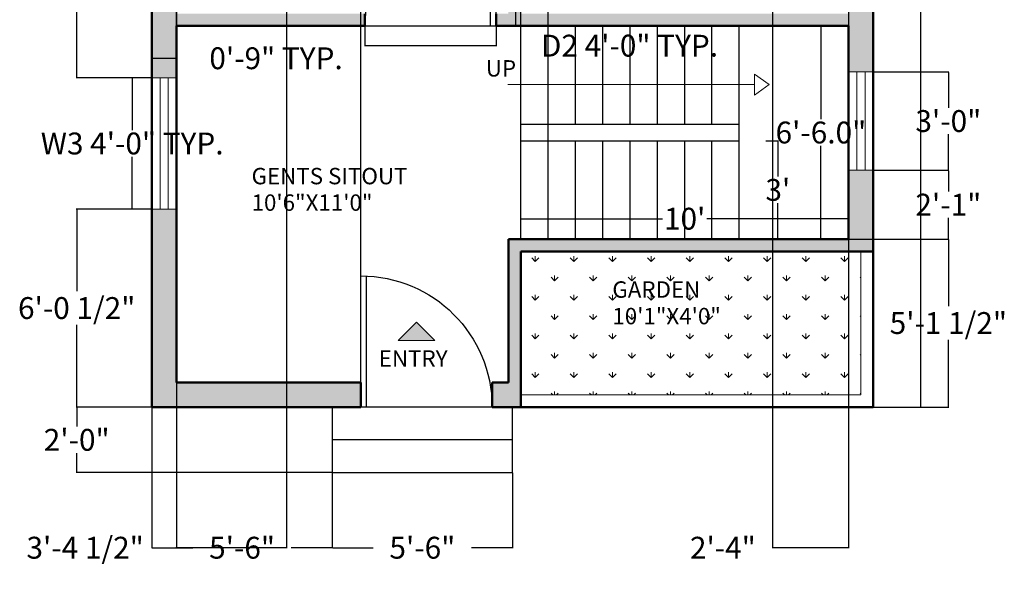
# Model space of a CAD drawing. Units: inches. Extents: x 23 to 387, y 67 to 650.
# Tile 1 of 3: x 23 to 384, y 67 to 272. Entities that reach past the tile are written whole.
import ezdxf

# ---------------------------------------------------------------- set-up
doc = ezdxf.new("R2010")
doc.units = ezdxf.units.IN
doc.header["$MEASUREMENT"] = 0
for name, color, linetype, lineweight in [('A-ANNO-DIMS', 4, 'Continuous', 18), ('A-ANNO-SYMB', 7, 'Continuous', 18), ('A-ANNO-TEXT', 4, 'Continuous', 18), ('A-AREA-IDEN', 4, 'Continuous', 25), ('A-DOOR', 41, 'Continuous', 25), ('A-FLOR-STRS', 215, 'Continuous', 25), ('A-GLAZ', 146, 'Continuous', 18), ('A-WALL', 240, 'Continuous', 50), ('A-WALL-PATT', 31, 'Continuous', 13), ('L-PLNT', 85, 'Continuous', 18), ('L-PLNT-PATT', 114, 'Continuous', 13)]:
    doc.layers.add(name, color=color, linetype=linetype, lineweight=lineweight)
doc.styles.get("Standard").update_dxf_attribs({"font": 'italic8.shx'})
doc.dimstyles.get("Standard").update_dxf_attribs({"dimtxt": 8, "dimasz": 0.18, "dimexe": 0.18, "dimexo": 0.0625, "dimgap": 0.09, "dimtad": 0, "dimtih": 1, "dimtoh": 1, "dimdec": 1, "dimzin": 0, "dimdsep": 46, "dimlunit": 3, "dimtxsty": 'Standard', "dimcen": 0.09, "dimadec": 0, "dimazin": 0, "dimtfac": 1, "dimtdec": 1, "dimtofl": 0, "dimtmove": 0, "dimatfit": 3, "dimfxl": 1, "dimtolj": 1, "dimtzin": 0, "dimarcsym": 0})

# ---------------------------------------------------------------- blocks, each defined once
blk = doc.blocks.new('*D1')
at = {"layer": 'A-ANNO-DIMS', "color": 0, "lineweight": -2, "transparency": 16777216}
for p, q in [((206.8, 199.3), (206.8, 199.68)), ((206.98, 199.5), (258.71, 199.5)), ((326.62, 199.5), (274.89, 199.5)), ((326.8, 199.3), (326.8, 199.68))]:
    blk.add_line(p, q, dxfattribs=at)
at = {"layer": 'A-ANNO-DIMS', "color": 0, "transparency": 16777216}
for points in [[(206.98, 199.53), (206.98, 199.47), (206.8, 199.5)], [(326.62, 199.53), (326.62, 199.47), (326.8, 199.5)]]:
    blk.add_solid(points, dxfattribs=at)
at = {"layer": 'Defpoints', "color": 0, "transparency": 16777216}
for p in [(206.8, 199.5), (206.8, 199.23), (326.8, 199.23)]:
    blk.add_point(p, dxfattribs=at)
at = {"layer": 'A-ANNO-DIMS', "color": 0, "transparency": 16777216, "insert": (266.8, 199.5), "char_height": 8, "attachment_point": 5}
blk.add_mtext("\\A1;10'", dxfattribs=at)
blk = doc.blocks.new('*D2')
at = {"layer": 'A-ANNO-DIMS', "color": 0, "lineweight": -2, "transparency": 16777216}
for p, q in [((316.66, 269.87), (316.66, 235.9)), ((316.72, 270.05), (316.84, 270.05)), ((316.66, 192.23), (316.66, 226.2)), ((316.72, 192.05), (316.84, 192.05))]:
    blk.add_line(p, q, dxfattribs=at)
at = {"layer": 'A-ANNO-DIMS', "color": 0, "transparency": 16777216}
for points in [[(316.63, 269.87), (316.69, 269.87), (316.66, 270.05)], [(316.63, 192.23), (316.69, 192.23), (316.66, 192.05)]]:
    blk.add_solid(points, dxfattribs=at)
at = {"layer": 'Defpoints', "color": 0, "transparency": 16777216}
for p in [(316.66, 270.05), (316.66, 270.05), (316.66, 192.05)]:
    blk.add_point(p, dxfattribs=at)
at = {"layer": 'A-ANNO-DIMS', "color": 0, "transparency": 16777216, "insert": (316.66, 231.05), "char_height": 8, "attachment_point": 5}
blk.add_mtext('\\A1;6\'-6.0"', dxfattribs=at)
blk = doc.blocks.new('*D3')
at = {"layer": 'A-ANNO-DIMS', "color": 0, "lineweight": -2, "transparency": 16777216}
for p, q in [((296.5, 228.05), (301.08, 228.05)), ((300.9, 227.87), (300.9, 214.9)), ((300.9, 192.23), (300.9, 205.2)), ((296.5, 192.05), (301.08, 192.05))]:
    blk.add_line(p, q, dxfattribs=at)
at = {"layer": 'A-ANNO-DIMS', "color": 0, "transparency": 16777216}
for points in [[(300.87, 227.87), (300.93, 227.87), (300.9, 228.05)], [(300.87, 192.23), (300.93, 192.23), (300.9, 192.05)]]:
    blk.add_solid(points, dxfattribs=at)
at = {"layer": 'Defpoints', "color": 0, "transparency": 16777216}
for p in [(296.44, 228.05), (300.9, 228.05), (296.44, 192.05)]:
    blk.add_point(p, dxfattribs=at)
at = {"layer": 'A-ANNO-DIMS', "color": 0, "transparency": 16777216, "insert": (300.9, 210.05), "char_height": 8, "attachment_point": 5}
blk.add_mtext("\\A1;3'", dxfattribs=at)
blk = doc.blocks.new('*D5')
at = {"layer": 'A-ANNO-DIMS', "color": 0, "lineweight": -2, "transparency": 16777216}
for p, q in [((335.86, 610.55), (353.42, 610.55)), ((353.24, 610.37), (353.24, 375.4)), ((353.24, 130.73), (353.24, 365.7)), ((335.86, 130.55), (353.42, 130.55))]:
    blk.add_line(p, q, dxfattribs=at)
at = {"layer": 'A-ANNO-DIMS', "color": 0, "transparency": 16777216}
for points in [[(353.21, 610.37), (353.27, 610.37), (353.24, 610.55)], [(353.21, 130.73), (353.27, 130.73), (353.24, 130.55)]]:
    blk.add_solid(points, dxfattribs=at)
at = {"layer": 'Defpoints', "color": 0, "transparency": 16777216}
for p in [(335.8, 610.55), (335.8, 130.55), (353.24, 130.55)]:
    blk.add_point(p, dxfattribs=at)
at = {"layer": 'A-ANNO-DIMS', "color": 0, "transparency": 16777216, "insert": (353.24, 370.55), "char_height": 8, "attachment_point": 5}
blk.add_mtext("\\A1;40'", dxfattribs=at)
blk = doc.blocks.new('DOOR-SWING-48IN')
for p, q in [((46, 0), (46, 47.96)), ((48, 0), (48, 48)), ((0, 0), (48, 0))]:
    blk.add_line(p, q)
blk.add_arc((48, 0), 48, 90, 180)
blk = doc.blocks.new('WIN-48IN')
for p, q in [((0, 0), (0, 48)), ((0, 48), (9, 48)), ((3, 0), (3, 48)), ((6, 0), (6, 48)), ((9, 48), (9, 0)), ((9, 0), (0, 0)), ((0, 0), (4.5, 0))]:
    blk.add_line(p, q)
blk = doc.blocks.new('*D16')
at = {"layer": 'A-ANNO-DIMS', "color": 0, "lineweight": -2, "transparency": 16777216}
for p, q in [((71.74, 251.04), (64.42, 251.04)), ((64.6, 250.86), (64.6, 231.89)), ((64.6, 203.22), (64.6, 222.19)), ((71.74, 203.04), (64.42, 203.04))]:
    blk.add_line(p, q, dxfattribs=at)
at = {"layer": 'A-ANNO-DIMS', "color": 0, "transparency": 16777216}
for points in [[(64.57, 250.86), (64.63, 250.86), (64.6, 251.04)], [(64.57, 203.22), (64.63, 203.22), (64.6, 203.04)]]:
    blk.add_solid(points, dxfattribs=at)
at = {"layer": 'Defpoints', "color": 0, "transparency": 16777216}
for p in [(64.6, 251.04), (71.8, 251.04), (71.8, 203.04)]:
    blk.add_point(p, dxfattribs=at)
at = {"layer": 'A-ANNO-DIMS', "color": 0, "transparency": 16777216, "insert": (64.6, 227.04), "char_height": 8, "attachment_point": 5}
blk.add_mtext('\\A1;W3 4\'-0" TYP.', dxfattribs=at)
blk = doc.blocks.new('*D17')
at = {"layer": 'A-ANNO-DIMS', "color": 0, "lineweight": -2, "transparency": 16777216}
for p, q in [((71.8, 251.1), (71.8, 258.42)), ((71.98, 258.24), (80.62, 258.24)), ((80.8, 251.1), (80.8, 258.42)), ((80.8, 258.24), (80.98, 258.24))]:
    blk.add_line(p, q, dxfattribs=at)
at = {"layer": 'A-ANNO-DIMS', "color": 0, "transparency": 16777216}
for points in [[(71.98, 258.27), (71.98, 258.21), (71.8, 258.24)], [(80.62, 258.27), (80.62, 258.21), (80.8, 258.24)]]:
    blk.add_solid(points, dxfattribs=at)
at = {"layer": 'Defpoints', "color": 0, "transparency": 16777216}
for p in [(80.8, 258.24), (71.8, 251.04), (80.8, 251.04)]:
    blk.add_point(p, dxfattribs=at)
at = {"layer": 'A-ANNO-DIMS', "color": 0, "transparency": 16777216, "insert": (117.26, 258.24), "char_height": 8, "attachment_point": 5}
blk.add_mtext('\\A1;0\'-9" TYP.', dxfattribs=at)
blk = doc.blocks.new('*D22')
at = {"layer": 'A-ANNO-DIMS', "color": 0, "lineweight": -2, "transparency": 16777216}
for p, q in [((149.76, 269.99), (149.76, 262.67)), ((197.76, 269.99), (197.76, 262.67)), ((149.94, 262.85), (197.58, 262.85)), ((197.76, 262.85), (197.94, 262.85))]:
    blk.add_line(p, q, dxfattribs=at)
at = {"layer": 'A-ANNO-DIMS', "color": 0, "transparency": 16777216}
for points in [[(149.94, 262.88), (149.94, 262.82), (149.76, 262.85)], [(197.58, 262.88), (197.58, 262.82), (197.76, 262.85)]]:
    blk.add_solid(points, dxfattribs=at)
at = {"layer": 'Defpoints', "color": 0, "transparency": 16777216}
for p in [(149.76, 270.05), (197.76, 270.05), (197.76, 262.85)]:
    blk.add_point(p, dxfattribs=at)
at = {"layer": 'A-ANNO-DIMS', "color": 0, "transparency": 16777216, "insert": (246.6, 262.85), "char_height": 8, "attachment_point": 5}
blk.add_mtext('\\A1;D2 4\'-0" TYP.', dxfattribs=at)
blk = doc.blocks.new('*D23')
at = {"layer": 'A-ANNO-DIMS', "color": 0, "lineweight": -2, "transparency": 16777216}
for p, q in [((197.82, 318.05), (205.14, 318.05)), ((204.96, 317.87), (204.96, 298.9)), ((204.96, 270.23), (204.96, 289.2)), ((197.82, 270.05), (205.14, 270.05))]:
    blk.add_line(p, q, dxfattribs=at)
at = {"layer": 'A-ANNO-DIMS', "color": 0, "transparency": 16777216}
for points in [[(204.93, 317.87), (204.99, 317.87), (204.96, 318.05)], [(204.93, 270.23), (204.99, 270.23), (204.96, 270.05)]]:
    blk.add_solid(points, dxfattribs=at)
at = {"layer": 'Defpoints', "color": 0, "transparency": 16777216}
for p in [(197.76, 318.05), (204.96, 318.05), (197.76, 270.05)]:
    blk.add_point(p, dxfattribs=at)
at = {"layer": 'A-ANNO-DIMS', "color": 0, "transparency": 16777216, "insert": (204.96, 294.05), "char_height": 8, "attachment_point": 5}
blk.add_mtext('\\A1;4\'-0" TYP.', dxfattribs=at)
blk = doc.blocks.new('*D24')
at = {"layer": 'A-ANNO-DIMS', "color": 0, "lineweight": -2, "transparency": 16777216}
for p, q in [((71.74, 130.55), (44.12, 130.55)), ((44.3, 130.37), (44.3, 123.4)), ((44.3, 106.73), (44.3, 113.7)), ((137.77, 106.55), (44.12, 106.55))]:
    blk.add_line(p, q, dxfattribs=at)
at = {"layer": 'A-ANNO-DIMS', "color": 0, "transparency": 16777216}
for points in [[(44.27, 130.37), (44.33, 130.37), (44.3, 130.55)], [(44.27, 106.73), (44.33, 106.73), (44.3, 106.55)]]:
    blk.add_solid(points, dxfattribs=at)
at = {"layer": 'Defpoints', "color": 0, "transparency": 16777216}
for p in [(44.3, 130.55), (71.8, 130.55), (137.83, 106.55)]:
    blk.add_point(p, dxfattribs=at)
at = {"layer": 'A-ANNO-DIMS', "color": 0, "transparency": 16777216, "insert": (44.3, 118.55), "char_height": 8, "attachment_point": 5}
blk.add_mtext('\\A1;2\'-0"', dxfattribs=at)
blk = doc.blocks.new('*D25')
at = {"layer": 'A-ANNO-DIMS', "color": 0, "lineweight": -2, "transparency": 16777216}
for p, q in [((137.83, 106.49), (137.83, 78.87)), ((203.79, 106.49), (203.79, 78.87)), ((138.01, 79.05), (152.81, 79.05)), ((203.61, 79.05), (188.8, 79.05))]:
    blk.add_line(p, q, dxfattribs=at)
at = {"layer": 'A-ANNO-DIMS', "color": 0, "transparency": 16777216}
for points in [[(138.01, 79.08), (138.01, 79.02), (137.83, 79.05)], [(203.61, 79.08), (203.61, 79.02), (203.79, 79.05)]]:
    blk.add_solid(points, dxfattribs=at)
at = {"layer": 'Defpoints', "color": 0, "transparency": 16777216}
for p in [(137.83, 106.55), (203.79, 106.55), (203.79, 79.05)]:
    blk.add_point(p, dxfattribs=at)
at = {"layer": 'A-ANNO-DIMS', "color": 0, "transparency": 16777216, "insert": (170.81, 79.05), "char_height": 8, "attachment_point": 5}
blk.add_mtext('\\A1;5\'-6"', dxfattribs=at)
blk = doc.blocks.new('*D26')
at = {"layer": 'A-ANNO-DIMS', "color": 0, "lineweight": -2, "transparency": 16777216}
for p, q in [((71.8, 130.49), (71.8, 78.87)), ((137.83, 106.49), (137.83, 78.87)), ((71.98, 79.05), (86.82, 79.05)), ((137.65, 79.05), (122.81, 79.05))]:
    blk.add_line(p, q, dxfattribs=at)
at = {"layer": 'A-ANNO-DIMS', "color": 0, "transparency": 16777216}
for points in [[(71.98, 79.08), (71.98, 79.02), (71.8, 79.05)], [(137.65, 79.08), (137.65, 79.02), (137.83, 79.05)]]:
    blk.add_solid(points, dxfattribs=at)
at = {"layer": 'Defpoints', "color": 0, "transparency": 16777216}
for p in [(71.8, 130.55), (137.83, 106.55), (137.83, 79.05)]:
    blk.add_point(p, dxfattribs=at)
at = {"layer": 'A-ANNO-DIMS', "color": 0, "transparency": 16777216, "insert": (104.82, 79.05), "char_height": 8, "attachment_point": 5}
blk.add_mtext('\\A1;5\'-6"', dxfattribs=at)
blk = doc.blocks.new('*D28')
at = {"layer": 'A-ANNO-DIMS', "color": 0, "lineweight": -2, "transparency": 16777216}
for p, q in [((71.74, 203.04), (44.12, 203.04)), ((44.3, 202.86), (44.3, 172.98)), ((44.3, 130.73), (44.3, 160.61)), ((71.74, 130.55), (44.12, 130.55))]:
    blk.add_line(p, q, dxfattribs=at)
at = {"layer": 'A-ANNO-DIMS', "color": 0, "transparency": 16777216}
for points in [[(44.27, 202.86), (44.33, 202.86), (44.3, 203.04)], [(44.27, 130.73), (44.33, 130.73), (44.3, 130.55)]]:
    blk.add_solid(points, dxfattribs=at)
at = {"layer": 'Defpoints', "color": 0, "transparency": 16777216}
for p in [(44.3, 203.04), (71.8, 203.04), (71.8, 130.55)]:
    blk.add_point(p, dxfattribs=at)
at = {"layer": 'A-ANNO-DIMS', "color": 0, "transparency": 16777216, "insert": (44.3, 166.79), "char_height": 8, "attachment_point": 5}
blk.add_mtext('\\A1;6\'-0 1/2"', dxfattribs=at)
blk = doc.blocks.new('*D31')
at = {"layer": 'A-ANNO-DIMS', "color": 0, "lineweight": -2, "transparency": 16777216}
for p, q in [((71.74, 322.2), (44.12, 322.2)), ((44.3, 322.02), (44.3, 291.47)), ((44.3, 251.22), (44.3, 281.76)), ((71.74, 251.04), (44.12, 251.04))]:
    blk.add_line(p, q, dxfattribs=at)
at = {"layer": 'A-ANNO-DIMS', "color": 0, "transparency": 16777216}
for points in [[(44.27, 322.02), (44.33, 322.02), (44.3, 322.2)], [(44.27, 251.22), (44.33, 251.22), (44.3, 251.04)]]:
    blk.add_solid(points, dxfattribs=at)
at = {"layer": 'Defpoints', "color": 0, "transparency": 16777216}
for p in [(71.8, 322.2), (44.3, 251.04), (71.8, 251.04)]:
    blk.add_point(p, dxfattribs=at)
at = {"layer": 'A-ANNO-DIMS', "color": 0, "transparency": 16777216, "insert": (44.3, 286.62), "char_height": 8, "attachment_point": 5}
blk.add_mtext('\\A1;5\'-11"', dxfattribs=at)
blk = doc.blocks.new('*D32')
at = {"layer": 'A-ANNO-DIMS', "color": 0, "lineweight": -2, "transparency": 16777216}
for p, q in [((335.86, 217.25), (363.48, 217.25)), ((363.3, 217.07), (363.3, 209.5)), ((363.3, 192.23), (363.3, 199.8)), ((326.86, 192.05), (363.48, 192.05))]:
    blk.add_line(p, q, dxfattribs=at)
at = {"layer": 'A-ANNO-DIMS', "color": 0, "transparency": 16777216}
for points in [[(363.27, 217.07), (363.33, 217.07), (363.3, 217.25)], [(363.27, 192.23), (363.33, 192.23), (363.3, 192.05)]]:
    blk.add_solid(points, dxfattribs=at)
at = {"layer": 'Defpoints', "color": 0, "transparency": 16777216}
for p in [(335.8, 217.25), (363.3, 217.25), (326.8, 192.05)]:
    blk.add_point(p, dxfattribs=at)
at = {"layer": 'A-ANNO-DIMS', "color": 0, "transparency": 16777216, "insert": (363.3, 204.65), "char_height": 8, "attachment_point": 5}
blk.add_mtext('\\A1;2\'-1"', dxfattribs=at)
blk = doc.blocks.new('*D36')
at = {"layer": 'A-ANNO-DIMS', "color": 0, "lineweight": -2, "transparency": 16777216}
for p, q in [((335.86, 253.25), (363.48, 253.25)), ((363.3, 253.07), (363.3, 240.11)), ((363.3, 217.43), (363.3, 230.4)), ((335.86, 217.25), (363.48, 217.25))]:
    blk.add_line(p, q, dxfattribs=at)
at = {"layer": 'A-ANNO-DIMS', "color": 0, "transparency": 16777216}
for points in [[(363.27, 253.07), (363.33, 253.07), (363.3, 253.25)], [(363.27, 217.43), (363.33, 217.43), (363.3, 217.25)]]:
    blk.add_solid(points, dxfattribs=at)
at = {"layer": 'Defpoints', "color": 0, "transparency": 16777216}
for p in [(335.8, 253.25), (335.8, 217.25), (363.3, 217.25)]:
    blk.add_point(p, dxfattribs=at)
at = {"layer": 'A-ANNO-DIMS', "color": 0, "transparency": 16777216, "insert": (363.3, 235.25), "char_height": 8, "attachment_point": 5}
blk.add_mtext('\\A1;3\'-0"', dxfattribs=at)
blk = doc.blocks.new('*D37')
at = {"layer": 'A-ANNO-DIMS', "color": 0, "lineweight": -2, "transparency": 16777216}
for p, q in [((80.8, 139.61), (80.8, 638.23)), ((80.98, 638.05), (81.51, 638.05)), ((148.12, 638.05), (147.59, 638.05)), ((148.3, 139.61), (148.3, 638.23))]:
    blk.add_line(p, q, dxfattribs=at)
at = {"layer": 'A-ANNO-DIMS', "color": 0, "transparency": 16777216}
for points in [[(80.98, 638.08), (80.98, 638.02), (80.8, 638.05)], [(148.12, 638.08), (148.12, 638.02), (148.3, 638.05)]]:
    blk.add_solid(points, dxfattribs=at)
at = {"layer": 'Defpoints', "color": 0, "transparency": 16777216}
for p in [(148.3, 638.05), (80.8, 139.55), (148.3, 139.55)]:
    blk.add_point(p, dxfattribs=at)
at = {"layer": 'A-ANNO-DIMS', "color": 0, "transparency": 16777216, "insert": (114.55, 638.05), "char_height": 8, "attachment_point": 5}
blk.add_mtext('\\A1;5\'-7 1/2"', dxfattribs=at)
blk = doc.blocks.new('*D39')
at = {"layer": 'A-ANNO-DIMS', "color": 0, "lineweight": -2, "transparency": 16777216}
for p, q in [((206.8, 192.11), (206.8, 638.23)), ((206.98, 638.05), (216.62, 638.05)), ((216.8, 192.11), (216.8, 638.23)), ((216.8, 638.05), (216.98, 638.05))]:
    blk.add_line(p, q, dxfattribs=at)
at = {"layer": 'A-ANNO-DIMS', "color": 0, "transparency": 16777216}
for points in [[(206.98, 638.08), (206.98, 638.02), (206.8, 638.05)], [(216.62, 638.08), (216.62, 638.02), (216.8, 638.05)]]:
    blk.add_solid(points, dxfattribs=at)
at = {"layer": 'Defpoints', "color": 0, "transparency": 16777216}
for p in [(216.8, 638.05), (206.8, 192.05), (216.8, 192.05)]:
    blk.add_point(p, dxfattribs=at)
at = {"layer": 'A-ANNO-DIMS', "color": 0, "transparency": 16777216, "insert": (237.64, 638.05), "char_height": 8, "attachment_point": 5}
blk.add_mtext('\\A1;0\'-10"', dxfattribs=at)
blk = doc.blocks.new('*D40')
at = {"layer": 'A-ANNO-DIMS', "color": 0, "lineweight": -2, "transparency": 16777216}
for p, q in [((80.8, 601.49), (80.8, 78.87)), ((121.14, 558.4), (121.14, 78.87)), ((80.8, 79.05), (80.62, 79.05)), ((120.96, 79.05), (80.98, 79.05))]:
    blk.add_line(p, q, dxfattribs=at)
at = {"layer": 'A-ANNO-DIMS', "color": 0, "transparency": 16777216}
for points in [[(80.98, 79.08), (80.98, 79.02), (80.8, 79.05)], [(120.96, 79.08), (120.96, 79.02), (121.14, 79.05)]]:
    blk.add_solid(points, dxfattribs=at)
at = {"layer": 'Defpoints', "color": 0, "transparency": 16777216}
for p in [(80.8, 601.55), (121.14, 558.46), (80.8, 79.05)]:
    blk.add_point(p, dxfattribs=at)
at = {"layer": 'A-ANNO-DIMS', "color": 0, "transparency": 16777216, "insert": (47.39, 79.05), "char_height": 8, "attachment_point": 5}
blk.add_mtext('\\A1;3\'-4 1/2"', dxfattribs=at)
blk = doc.blocks.new('*D43')
at = {"layer": 'A-ANNO-DIMS', "color": 0, "lineweight": -2, "transparency": 16777216}
for p, q in [((326.8, 601.49), (326.8, 78.87)), ((298.95, 586.36), (298.95, 78.87)), ((298.95, 79.05), (298.77, 79.05)), ((326.62, 79.05), (299.13, 79.05))]:
    blk.add_line(p, q, dxfattribs=at)
at = {"layer": 'A-ANNO-DIMS', "color": 0, "transparency": 16777216}
for points in [[(299.13, 79.08), (299.13, 79.02), (298.95, 79.05)], [(326.62, 79.08), (326.62, 79.02), (326.8, 79.05)]]:
    blk.add_solid(points, dxfattribs=at)
at = {"layer": 'Defpoints', "color": 0, "transparency": 16777216}
for p in [(326.8, 601.55), (298.95, 586.43), (298.95, 79.05)]:
    blk.add_point(p, dxfattribs=at)
at = {"layer": 'A-ANNO-DIMS', "color": 0, "transparency": 16777216, "insert": (280.78, 79.05), "char_height": 8, "attachment_point": 5}
blk.add_mtext('\\A1;2\'-4"', dxfattribs=at)
blk = doc.blocks.new('*D47')
at = {"layer": 'A-ANNO-DIMS', "color": 0, "lineweight": -2, "transparency": 16777216}
for p, q in [((326.86, 192.05), (363.48, 192.05)), ((363.3, 191.87), (363.3, 167.48)), ((363.3, 130.73), (363.3, 155.11)), ((335.86, 130.55), (363.48, 130.55))]:
    blk.add_line(p, q, dxfattribs=at)
at = {"layer": 'A-ANNO-DIMS', "color": 0, "transparency": 16777216}
for points in [[(363.27, 191.87), (363.33, 191.87), (363.3, 192.05)], [(363.27, 130.73), (363.33, 130.73), (363.3, 130.55)]]:
    blk.add_solid(points, dxfattribs=at)
at = {"layer": 'Defpoints', "color": 0, "transparency": 16777216}
for p in [(326.8, 192.05), (363.3, 192.05), (335.8, 130.55)]:
    blk.add_point(p, dxfattribs=at)
at = {"layer": 'A-ANNO-DIMS', "color": 0, "transparency": 16777216, "insert": (363.3, 161.3), "char_height": 8, "attachment_point": 5}
blk.add_mtext('\\A1;5\'-1 1/2"', dxfattribs=at)

msp = doc.modelspace()

# ---------------------------------------------------------------- hatches: boundary and pattern name
at = {"layer": 'A-ANNO-SYMB'}
h = msp.add_hatch(color=256, dxfattribs=at)
h.dxf.hatch_style = 1
h.paths.add_polyline_path([(168.68, 161.67), (161.99, 154.96), (168.68, 154.96), (175.36, 154.96)])
at = {"layer": 'A-WALL-PATT'}
h = msp.add_hatch(color=256, dxfattribs=at)
h.dxf.hatch_style = 1
h.paths.add_polyline_path([(80.8, 601.55), (168.85, 601.55), (168.85, 610.55), (71.8, 610.55), (71.8, 559.71), (80.8, 559.71)])
h.paths.add_polyline_path([(335.8, 610.55), (198.85, 610.55), (198.85, 601.55), (202.3, 601.55), (202.3, 481.55), (202.3, 465.05), (207.59, 465.05), (207.59, 469.55), (206.8, 469.55), (206.8, 601.55), (326.8, 601.55), (326.8, 570), (331.3, 570), (335.8, 570)])
h.paths.add_polyline_path([(335.8, 510), (326.8, 510), (326.8, 469.55), (249.59, 469.55), (249.59, 465.05), (250.3, 465.05), (250.3, 461.06), (254.8, 461.06), (254.8, 465.05), (326.8, 465.05), (326.8, 455.49), (335.8, 455.49)])
h.paths.add_polyline_path([(335.8, 425.49), (326.8, 425.49), (326.8, 414.55), (254.8, 414.55), (254.8, 431.06), (250.3, 431.06), (250.3, 414.55), (249.82, 414.55), (249.82, 410.05), (326.8, 410.05), (326.8, 362.57), (335.8, 362.57)])
h.paths.add_polyline_path([(335.8, 302.57), (326.8, 302.57), (326.8, 274.55), (206.8, 274.55), (206.8, 410.05), (207.82, 410.05), (207.82, 414.55), (202.3, 414.55), (202.3, 274.55), (197.76, 274.55), (197.76, 270.05), (326.8, 270.05), (326.8, 253.25), (335.8, 253.25)])
h.paths.add_polyline_path([(335.8, 217.25), (326.8, 217.25), (326.8, 192.05), (202.3, 192.05), (202.3, 139.55), (196.3, 139.55), (196.3, 130.55), (206.8, 130.55), (206.8, 187.55), (335.8, 187.55)])
h.paths.add_polyline_path([(80.8, 203.04), (71.8, 203.04), (71.8, 130.55), (148.3, 130.55), (148.3, 139.55), (80.8, 139.55)])
h.paths.add_polyline_path([(80.8, 322.2), (71.8, 322.2), (71.8, 251.04), (80.8, 251.04), (80.8, 270.05), (149.76, 270.05), (149.76, 274.55), (80.8, 274.55)])
h.paths.add_polyline_path([(80.8, 410.05), (133.3, 410.05), (133.3, 433.95), (128.8, 433.95), (128.8, 414.55), (80.8, 414.55), (80.8, 426.74), (71.8, 426.74), (71.8, 382.2), (80.8, 382.2)])
h.paths.add_polyline_path([(133.3, 479.05), (80.8, 479.05), (80.8, 511.71), (71.8, 511.71), (71.8, 456.74), (80.8, 456.74), (80.8, 474.55), (128.8, 474.55), (128.8, 469.95), (133.3, 469.95)])
h.paths.add_polyline_path([(82.53, 419.2), (134.1, 419.2), (134.1, 429.92), (82.53, 429.92)], flags=9)
at = {"layer": 'L-PLNT-PATT'}
h = msp.add_hatch(dxfattribs=at)
h.set_pattern_fill('GRASS', color=256, scale=10)
h.paths.add_polyline_path([(331.3, 187.55), (206.8, 187.55), (206.8, 135.05), (331.3, 135.05)])
h.paths.add_polyline_path([(238.84, 159.07), (292.13, 159.07), (292.13, 169.78), (238.84, 169.78)], flags=24)
h.paths.add_polyline_path([(238.84, 169.07), (281.55, 169.07), (281.55, 178.07), (238.84, 178.07)], flags=24)

# ---------------------------------------------------------------- linework, layer by layer
at = {"layer": 'A-ANNO-SYMB'}
for p, q in [((292.34, 248.57), (292.34, 252.44)), ((292.34, 252.44), (297.7, 248.57)), ((202.08, 248.57), (292.34, 248.57)), ((292.34, 248.57), (292.34, 244.7)), ((292.34, 244.7), (297.7, 248.57)), ((161.99, 154.96), (168.68, 161.67)), ((175.36, 154.96), (168.68, 161.67)), ((168.68, 154.96), (161.99, 154.96)), ((168.68, 154.96), (175.36, 154.96))]:
    msp.add_line(p, q, dxfattribs=at)
at = {"layer": 'A-FLOR-STRS'}
for p, q in [((206.8, 192.05), (206.8, 270.05)), ((216.8, 234.05), (216.8, 270.05)), ((226.8, 234.05), (226.8, 270.05)), ((236.8, 234.05), (236.8, 270.05)), ((246.8, 234.05), (246.8, 270.05)), ((256.8, 234.05), (256.8, 270.05)), ((266.8, 234.05), (266.8, 270.05)), ((276.8, 234.05), (276.8, 270.05)), ((286.8, 192.05), (286.8, 270.05)), ((206.8, 234.05), (286.8, 234.05)), ((206.8, 228.05), (286.8, 228.05)), ((216.8, 192.05), (216.8, 228.05)), ((226.8, 192.05), (226.8, 228.05)), ((236.8, 192.05), (236.8, 228.05)), ((246.8, 192.05), (246.8, 228.05)), ((256.8, 192.05), (256.8, 228.05)), ((266.8, 192.05), (266.8, 228.05)), ((276.8, 192.05), (276.8, 228.05)), ((137.83, 130.55), (137.83, 106.55)), ((203.79, 106.55), (203.79, 130.55)), ((203.79, 118.55), (137.83, 118.55)), ((137.83, 106.55), (203.79, 106.55))]:
    msp.add_line(p, q, dxfattribs=at)
at = {"layer": 'A-GLAZ'}
for p, q in [((326.8, 217.25), (326.8, 253.25)), ((326.8, 253.25), (335.8, 253.25)), ((329.8, 217.25), (329.8, 253.25)), ((332.8, 217.25), (332.8, 253.25)), ((335.8, 253.25), (335.8, 217.25)), ((335.8, 217.25), (326.8, 217.25)), ((326.8, 217.25), (331.3, 217.25))]:
    msp.add_line(p, q, dxfattribs=at)
at = {"layer": 'A-WALL'}
for p, q in [((71.8, 610.55), (71.8, 130.55)), ((335.8, 130.55), (335.8, 610.55)), ((149.76, 274.55), (149.76, 270.05)), ((197.76, 274.55), (197.76, 270.05)), ((80.8, 270.05), (149.76, 270.05)), ((80.8, 270.05), (80.8, 139.55)), ((197.76, 270.05), (326.8, 270.05)), ((326.8, 192.05), (326.8, 270.05)), ((202.3, 139.55), (202.3, 192.05)), ((202.3, 192.05), (326.8, 192.05)), ((206.8, 130.55), (206.8, 187.55)), ((206.8, 187.55), (335.8, 187.55)), ((80.8, 139.55), (148.3, 139.55)), ((148.3, 139.55), (148.3, 130.55)), ((196.3, 139.55), (196.3, 130.55)), ((196.3, 139.55), (202.3, 139.55)), ((71.8, 130.55), (148.3, 130.55)), ((196.3, 130.55), (335.8, 130.55))]:
    msp.add_line(p, q, dxfattribs=at)
at = {"layer": 'L-PLNT'}
for p, q in [((331.3, 135.05), (331.3, 187.55)), ((206.8, 135.05), (331.3, 135.05))]:
    msp.add_line(p, q, dxfattribs=at)

# ---------------------------------------------------------------- block references
at = {"layer": 'A-DOOR'}
msp.add_blockref('DOOR-SWING-48IN', (149.76, 270.05), dxfattribs=at)
at = {"layer": 'A-DOOR', "extrusion": (0, 0, -1), "zscale": -1}
msp.add_blockref('DOOR-SWING-48IN', (-196.3, 130.55), dxfattribs=at)
at = {"layer": 'A-GLAZ'}
msp.add_blockref('WIN-48IN', (71.8, 203.04), dxfattribs=at)

# ---------------------------------------------------------------- texts
at = {"layer": 'A-ANNO-TEXT'}
for s, p in [('UP', (194.03, 251.54)), ('ENTRY', (154.85, 145.32))]:
    msp.add_text(s, height=6, dxfattribs=at).set_placement(p)
at = {"layer": 'A-AREA-IDEN'}
for s, p in [('GENTS SITOUT', (108.3, 212.1)), ('10\'6"X11\'0"', (108.3, 202.39)), ('GARDEN', (240.34, 170.57)), ('10\'1"X4\'0"', (240.34, 160.85))]:
    msp.add_text(s, height=6, dxfattribs=at).set_placement(p)

# ---------------------------------------------------------------- dimensions: what is measured, and where the dimension line sits
at = {"layer": 'A-ANNO-DIMS'}
for base, p1, p2, override, picture, middle in [((148.3, 638.05), (80.8, 139.55), (148.3, 139.55), {"dimdec": 1, "dimlfac": 1, "dimrnd": 0, "dimzin": 1, "dimdsep": 46, "dimlunit": 4, "dimfrac": 2}, '*D37', (114.55, 638.05)), ((216.8, 638.05), (206.8, 192.05), (216.8, 192.05), {"dimdec": 1, "dimlfac": 1, "dimrnd": 0, "dimzin": 1, "dimdsep": 46, "dimlunit": 4, "dimfrac": 2}, '*D39', (237.64, 638.05)), ((80.8, 79.05), (121.14, 558.46), (80.8, 601.55), {"dimdec": 1, "dimlfac": 1, "dimrnd": 0, "dimzin": 1, "dimdsep": 46, "dimlunit": 4, "dimfrac": 2}, '*D40', (47.39, 79.05)), ((298.9524, 79.049), (326.7992, 601.549), (298.9524, 586.4268), {"dimdec": 1, "dimlfac": 1, "dimrnd": 0, "dimzin": 1, "dimdsep": 46, "dimlunit": 4, "dimfrac": 2}, '*D43', (280.7776, 79.049)), ((206.8, 199.5), (326.8, 199.23), (206.8, 199.23), {"dimclrd": 0, "dimclre": 0, "dimclrt": 0}, '*D1', (266.8, 199.5)), ((137.83, 79.05), (71.8, 130.55), (137.83, 106.55), {"dimdec": 1, "dimlfac": 1, "dimrnd": 0, "dimzin": 1, "dimdsep": 46, "dimlunit": 4, "dimfrac": 2}, '*D26', (104.82, 79.05)), ((203.79, 79.05), (137.83, 106.55), (203.79, 106.55), {"dimdec": 1, "dimlfac": 1, "dimrnd": 0, "dimzin": 1, "dimdsep": 46, "dimlunit": 4, "dimfrac": 2}, '*D25', (170.81, 79.05))]:
    dim = msp.add_linear_dim(base=base, p1=p1, p2=p2, dimstyle='Standard', override=override, dxfattribs=at)
    dim.commit()
    dim.dimension.update_dxf_attribs({"geometry": picture, "text_midpoint": middle})
for base, p1, p2, override, picture, middle in [((353.24, 130.55), (335.8, 610.55), (335.8, 130.55), {"dimclrd": 0, "dimclre": 0, "dimclrt": 0}, '*D5', (353.24, 370.55)), ((44.3, 251.04), (71.8, 322.2), (71.8, 251.04), {"dimdec": 1, "dimlfac": 1, "dimrnd": 0, "dimzin": 1, "dimdsep": 46, "dimlunit": 4, "dimfrac": 2}, '*D31', (44.3, 286.62)), ((316.66, 270.05), (316.66, 192.05), (316.66, 270.05), {"dimclrd": 0, "dimclre": 0, "dimclrt": 0}, '*D2', (316.66, 231.05)), ((363.3, 217.25), (335.8, 253.25), (335.8, 217.25), {"dimdec": 1, "dimlfac": 1, "dimrnd": 0, "dimzin": 1, "dimdsep": 46, "dimlunit": 4, "dimfrac": 2}, '*D36', (363.3, 235.25)), ((300.9, 228.05), (296.44, 192.05), (296.44, 228.05), {"dimclrd": 0, "dimclre": 0, "dimclrt": 0}, '*D3', (300.9, 210.05)), ((363.3, 217.25), (326.8, 192.05), (335.8, 217.25), {"dimdec": 1, "dimlfac": 1, "dimrnd": 0, "dimzin": 1, "dimdsep": 46, "dimlunit": 4, "dimfrac": 2}, '*D32', (363.3, 204.65)), ((44.3, 203.04), (71.8, 130.55), (71.8, 203.04), {"dimdec": 1, "dimlfac": 1, "dimrnd": 0, "dimzin": 1, "dimdsep": 46, "dimlunit": 4, "dimfrac": 2}, '*D28', (44.3, 166.79)), ((363.3, 192.05), (335.8, 130.55), (326.8, 192.05), {"dimdec": 1, "dimlfac": 1, "dimrnd": 0, "dimzin": 1, "dimdsep": 46, "dimlunit": 4, "dimfrac": 2}, '*D47', (363.3, 161.3)), ((44.3, 130.55), (137.83, 106.55), (71.8, 130.55), {"dimdec": 1, "dimlfac": 1, "dimrnd": 0, "dimzin": 1, "dimdsep": 46, "dimlunit": 4, "dimfrac": 2}, '*D24', (44.3, 118.55))]:
    dim = msp.add_linear_dim(base=base, p1=p1, p2=p2, angle=90, dimstyle='Standard', override=override, dxfattribs=at)
    dim.commit()
    dim.dimension.update_dxf_attribs({"geometry": picture, "text_midpoint": middle})
for base, p1, p2, text, picture, middle in [((204.96, 318.05), (197.76, 270.05), (197.76, 318.05), '<> TYP.', '*D23', (204.96, 294.05)), ((64.6, 251.04), (71.8, 203.04), (71.8, 251.04), 'W3 <> TYP.', '*D16', (64.6, 227.04))]:
    dim = msp.add_linear_dim(base=base, p1=p1, p2=p2, angle=90, text=text, dimstyle='Standard', override={"dimdec": 1, "dimlfac": 1, "dimrnd": 0, "dimzin": 1, "dimdsep": 46, "dimlunit": 4, "dimfrac": 2}, dxfattribs=at)
    dim.commit()
    dim.dimension.update_dxf_attribs({"geometry": picture, "text_midpoint": middle})
for base, p1, p2, text, picture, middle in [((197.76, 262.85), (149.76, 270.05), (197.76, 270.05), 'D2 <> TYP.', '*D22', (246.6, 262.85)), ((80.8, 258.24), (71.8, 251.04), (80.8, 251.04), '<> TYP.', '*D17', (117.26, 258.24))]:
    dim = msp.add_linear_dim(base=base, p1=p1, p2=p2, text=text, dimstyle='Standard', override={"dimdec": 1, "dimlfac": 1, "dimrnd": 0, "dimzin": 1, "dimdsep": 46, "dimlunit": 4, "dimfrac": 2}, dxfattribs=at)
    dim.commit()
    dim.dimension.update_dxf_attribs({"geometry": picture, "text_midpoint": middle})

doc.saveas('drawing.dxf')
